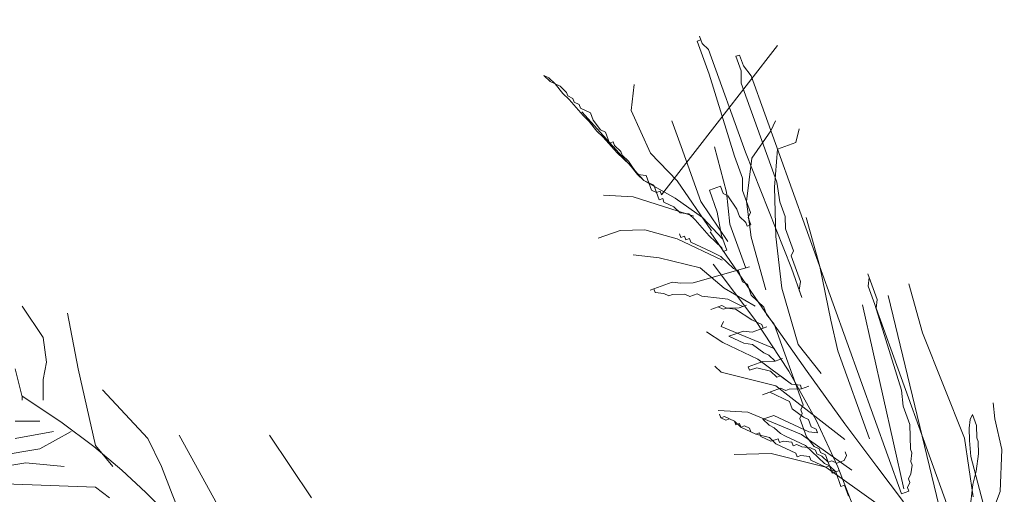
# Model space of a CAD drawing. Units: millimetres. Extents: x 595116 to 630915, y 909473 to 920225.
# Tile 73 of 134: x 629622.585 to 629629.81, y 919282.412 to 919285.898. Entities that reach past the tile are written whole.
import ezdxf

# ---------------------------------------------------------------- set-up
doc = ezdxf.new("R2010")
doc.units = ezdxf.units.MM
doc.layers.add('Dimension', color=3, linetype='Continuous', lineweight=18)
doc.layers.add('L-PLNT', color=85, linetype='Continuous', lineweight=13)
doc.styles.get("Standard").update_dxf_attribs({"font": 'arial.ttf'})
doc.dimstyles.new('ISO-25', dxfattribs={"dimtxt": 9, "dimasz": 6, "dimexe": 1.25, "dimexo": 0.625, "dimtad": 1, "dimlunit": 4, "dimtxsty": 'Standard', "dimcen": 2.5, "dimadec": 0, "dimazin": 0, "dimtfac": 1, "dimtmove": 0, "dimatfit": 3, "dimfxl": 1, "dimarcsym": 0})

# ---------------------------------------------------------------- blocks, each defined once
blk = doc.blocks.new('A$C4FB75ABC')
for p, q in [((2.2354, 4.7176), (2.2283, 4.715)), ((2.238, 4.7104), (2.2329, 4.7248)), ((2.2329, 4.7248), (2.2354, 4.7176)), ((2.1583, 4.4143), (2.3852, 4.7066)), ((2.2283, 4.715), (2.2515, 4.6504)), ((2.2504, 4.6987), (2.238, 4.7104)), ((2.3227, 4.4977), (2.2504, 4.6987)), ((2.3109, 4.688), (2.3037, 4.6854)), ((2.3037, 4.6854), (2.314, 4.6567)), ((2.3186, 4.6665), (2.3109, 4.688)), ((2.3336, 4.6475), (2.3186, 4.6665)), ((1.9382, 4.6431), (1.9285, 4.6477)), ((1.9285, 4.6477), (1.9408, 4.6359)), ((1.9506, 4.6313), (1.9382, 4.6431)), ((2.2515, 4.6504), (2.3011, 4.49)), ((2.314, 4.6567), (2.3146, 4.6326)), ((2.6279, 3.8295), (2.3336, 4.6475)), ((1.9408, 4.6359), (1.9506, 4.6313)), ((1.9603, 4.6267), (1.9506, 4.6313)), ((1.9506, 4.6313), (1.9655, 4.6124)), ((1.9726, 4.6149), (1.9603, 4.6267)), ((2.0989, 4.5793), (2.1049, 4.6301)), ((2.3146, 4.6326), (2.3843, 4.4389)), ((1.9655, 4.6124), (1.9778, 4.6006)), ((1.9752, 4.6078), (1.9726, 4.6149)), ((1.985, 4.6032), (1.9752, 4.6078)), ((1.9876, 4.596), (1.985, 4.6032)), ((1.9778, 4.6006), (2.0051, 4.5699)), ((1.9973, 4.5914), (1.9876, 4.596)), ((1.9999, 4.5842), (1.9973, 4.5914)), ((2.0097, 4.5796), (1.9999, 4.5842)), ((2.1238, 4.4424), (2.0025, 4.577)), ((2.0051, 4.5699), (2.0174, 4.5581)), ((2.0194, 4.575), (2.0097, 4.5796)), ((2.0246, 4.5607), (2.0194, 4.575)), ((2.137, 4.4958), (2.0989, 4.5793)), ((2.0174, 4.5581), (2.0323, 4.5391)), ((2.0395, 4.5417), (2.0246, 4.5607)), ((2.197, 4.5092), (2.1789, 4.5595)), ((2.3723, 4.5399), (2.3815, 4.5594)), ((2.4211, 4.5169), (2.4277, 4.5436)), ((2.0323, 4.5391), (2.0447, 4.5274)), ((2.0493, 4.5371), (2.0395, 4.5417)), ((2.0447, 4.5274), (2.0719, 4.4967)), ((2.057, 4.5156), (2.0493, 4.5371)), ((2.335, 4.486), (2.3723, 4.5399)), ((2.0642, 4.5182), (2.057, 4.5156)), ((2.0668, 4.511), (2.0642, 4.5182)), ((2.0791, 4.4992), (2.0668, 4.511)), ((2.2357, 4.4016), (2.197, 4.5092)), ((2.2859, 4.4197), (2.2621, 4.5084)), ((2.3852, 4.504), (2.4211, 4.5169)), ((2.0719, 4.4967), (2.0966, 4.4731)), ((2.0817, 4.4921), (2.0791, 4.4992)), ((2.094, 4.4803), (2.0817, 4.4921)), ((2.189, 4.4415), (2.137, 4.4958)), ((2.3011, 4.49), (2.3166, 4.4469)), ((2.4125, 4.2707), (2.3227, 4.4977)), ((2.325, 4.4013), (2.335, 4.486)), ((2.3797, 4.4291), (2.3852, 4.504)), ((2.1115, 4.4542), (2.094, 4.4803)), ((2.0966, 4.4731), (2.1115, 4.4542)), ((2.1238, 4.4424), (2.1115, 4.4542)), ((2.1115, 4.4542), (2.1284, 4.4522)), ((2.1284, 4.4522), (2.1336, 4.4378)), ((2.3166, 4.4469), (2.3172, 4.4228)), ((2.1336, 4.4378), (2.1238, 4.4424)), ((2.185, 4.4077), (2.1238, 4.4424)), ((2.1388, 4.4235), (2.1336, 4.4378)), ((2.1336, 4.4378), (2.1434, 4.4332)), ((2.1434, 4.4332), (2.1485, 4.4189)), ((2.2564, 4.3442), (2.189, 4.4415)), ((2.2736, 4.4314), (2.2521, 4.4237)), ((2.2788, 4.4171), (2.2736, 4.4314)), ((2.382, 4.3327), (2.3797, 4.4291)), ((2.3843, 4.4389), (2.3901, 4.4004)), ((2.1029, 4.4105), (2.0449, 4.414)), ((2.222, 4.3723), (2.1029, 4.4105)), ((2.1485, 4.4189), (2.1388, 4.4235)), ((2.1485, 4.4189), (2.1557, 4.4214)), ((2.1537, 4.4045), (2.1485, 4.4189)), ((2.1557, 4.4214), (2.1583, 4.4143)), ((2.2521, 4.4237), (2.2676, 4.3807)), ((2.2885, 4.4125), (2.2788, 4.4171)), ((2.2922, 4.3571), (2.2859, 4.4197)), ((2.306, 4.3864), (2.2885, 4.4125)), ((2.3172, 4.4228), (2.3327, 4.3798)), ((2.1609, 4.4071), (2.1537, 4.4045)), ((2.1634, 4.3999), (2.1609, 4.4071)), ((2.1829, 4.3907), (2.1634, 4.3999)), ((2.1953, 4.379), (2.1829, 4.3907)), ((2.2389, 4.3703), (2.185, 4.4077)), ((2.2882, 4.3232), (2.2357, 4.4016)), ((2.3338, 4.3316), (2.325, 4.4013)), ((2.3901, 4.4004), (2.4004, 4.3717)), ((2.2122, 4.3769), (2.1953, 4.379)), ((2.2245, 4.3652), (2.2122, 4.3769)), ((2.2785, 4.3278), (2.2389, 4.3703)), ((2.2676, 4.3807), (2.2759, 4.335)), ((2.3112, 4.372), (2.306, 4.3864)), ((2.3235, 4.3603), (2.3112, 4.372)), ((2.3327, 4.3798), (2.3281, 4.37)), ((2.3281, 4.37), (2.3333, 4.3557)), ((2.4004, 4.3717), (2.401, 4.3476)), ((2.4678, 4.2744), (2.4414, 4.3703)), ((2.2518, 4.3344), (2.2245, 4.3652)), ((2.3232, 4.271), (2.2922, 4.3571)), ((2.3261, 4.3531), (2.3235, 4.3603)), ((2.3333, 4.3557), (2.3261, 4.3531)), ((2.0779, 4.3448), (2.0349, 4.3293)), ((2.1261, 4.346), (2.0779, 4.3448)), ((2.1893, 4.3282), (2.1261, 4.346)), ((2.1938, 4.3379), (2.1964, 4.3307)), ((2.1964, 4.3307), (2.2036, 4.3333)), ((2.2036, 4.3333), (2.2062, 4.3261)), ((2.2641, 4.3227), (2.2518, 4.3344)), ((2.2538, 4.3417), (2.3557, 4.1924)), ((2.2759, 4.335), (2.2862, 4.3063)), ((2.3628, 4.2285), (2.3338, 4.3316)), ((2.3941, 4.2317), (2.382, 4.3327)), ((2.401, 4.3476), (2.4165, 4.3046)), ((2.277, 4.2868), (2.1893, 4.3282)), ((2.2062, 4.3261), (2.2134, 4.3287)), ((2.2134, 4.3287), (2.2159, 4.3215)), ((2.2159, 4.3215), (2.2354, 4.3124)), ((2.2354, 4.3124), (2.2452, 4.3078)), ((2.2765, 4.3109), (2.2641, 4.3227)), ((2.154, 4.2911), (2.1032, 4.2972)), ((2.2452, 4.3078), (2.255, 4.3032)), ((2.255, 4.3032), (2.2745, 4.294)), ((2.2745, 4.294), (2.2868, 4.2822)), ((2.2791, 4.3037), (2.2765, 4.3109)), ((2.2862, 4.3063), (2.2791, 4.3037)), ((2.4165, 4.3046), (2.4119, 4.2948)), ((2.4119, 4.2948), (2.43, 4.2446)), ((2.234, 4.2713), (2.154, 4.2911)), ((2.3407, 4.1707), (2.2593, 4.2788)), ((2.2868, 4.2822), (2.2991, 4.2704)), ((2.4896, 4.1688), (2.4678, 4.2744)), ((2.2202, 4.242), (2.3304, 4.2736)), ((2.2808, 4.2314), (2.234, 4.2713)), ((2.2991, 4.2704), (2.3089, 4.2658)), ((2.3089, 4.2658), (2.3166, 4.2443)), ((2.4331, 4.2133), (2.4125, 4.2707)), ((2.5803, 4.2095), (2.5622, 4.2597)), ((2.5622, 4.2597), (2.5648, 4.2526)), ((2.1362, 4.228), (2.1792, 4.2435)), ((2.1792, 4.2435), (2.1961, 4.2415)), ((2.1961, 4.2415), (2.2202, 4.242)), ((2.3166, 4.2443), (2.3264, 4.2397)), ((2.3264, 4.2397), (2.3341, 4.2182)), ((2.43, 4.2446), (2.4279, 4.2276)), ((2.5648, 4.2526), (2.5628, 4.2356)), ((2.5628, 4.2356), (2.5757, 4.1997)), ((2.6686, 4.144), (2.6423, 4.2399)), ((2.1434, 4.2306), (2.1362, 4.228)), ((2.1459, 4.2234), (2.1434, 4.2306)), ((2.1629, 4.2214), (2.1459, 4.2234)), ((2.1726, 4.2168), (2.1629, 4.2214)), ((2.1798, 4.2194), (2.1726, 4.2168)), ((2.2039, 4.22), (2.1798, 4.2194)), ((2.2136, 4.2154), (2.2039, 4.22)), ((2.228, 4.2205), (2.2136, 4.2154)), ((2.2377, 4.2159), (2.228, 4.2205)), ((2.2716, 4.2119), (2.2377, 4.2159)), ((2.3419, 4.1967), (2.2808, 4.2314)), ((2.3341, 4.2182), (2.3465, 4.2064)), ((2.4257, 4.1214), (2.3941, 4.2317)), ((2.4279, 4.2276), (2.4331, 4.2133)), ((2.7169, 3.7399), (2.6018, 4.2172)), ((2.2552, 4.1898), (2.2768, 4.1975)), ((2.2885, 4.2099), (2.2716, 4.2119)), ((2.2768, 4.1975), (2.2865, 4.1929)), ((2.308, 4.2007), (2.2885, 4.2099)), ((2.3178, 4.1961), (2.308, 4.2007)), ((2.3106, 4.1935), (2.325, 4.1987)), ((2.325, 4.1987), (2.3178, 4.1961)), ((2.3465, 4.2064), (2.3588, 4.1946)), ((2.6325, 3.8393), (2.5516, 4.1992)), ((2.5757, 4.1997), (2.6279, 4.0321)), ((2.5783, 4.1926), (2.5803, 4.2095)), ((0.9087, 4.1962), (0.9496, 4.1349)), ((0.9973, 4.1826), (1.0177, 4.0736)), ((2.2696, 4.195), (2.2552, 4.1898)), ((2.2793, 4.1904), (2.2696, 4.195)), ((2.2865, 4.1929), (2.2793, 4.1904)), ((2.2865, 4.1929), (2.3106, 4.1935)), ((2.3034, 4.1909), (2.2865, 4.1929)), ((2.3353, 4.17), (2.3034, 4.1909)), ((2.3557, 4.1924), (2.443, 4.0685)), ((2.3588, 4.1946), (2.364, 4.1803)), ((2.364, 4.1803), (2.3789, 4.1614)), ((2.8029, 3.5683), (2.5783, 4.1926)), ((2.2753, 4.1565), (2.2799, 4.1663)), ((2.345, 4.1654), (2.3353, 4.17)), ((2.4072, 4.0691), (2.3407, 4.1707)), ((2.3548, 4.1608), (2.345, 4.1654)), ((2.3574, 4.1536), (2.3548, 4.1608)), ((2.3789, 4.1614), (2.4357, 4.0035)), ((2.5031, 4.1088), (2.4896, 4.1688)), ((2.2785, 4.1252), (2.2466, 4.1462)), ((2.38, 4.1131), (2.2753, 4.1565)), ((2.2902, 4.1376), (2.3189, 4.1479)), ((2.3189, 4.1479), (2.3359, 4.1459)), ((2.3359, 4.1459), (2.3645, 4.1562)), ((2.3645, 4.1562), (2.3574, 4.1536)), ((2.7507, 3.9385), (2.6686, 4.144)), ((0.9496, 4.1349), (0.9564, 4.0872)), ((2.3468, 4.0931), (2.2785, 4.1252)), ((2.3, 4.133), (2.2902, 4.1376)), ((2.3098, 4.1284), (2.3, 4.133)), ((2.3195, 4.1238), (2.3098, 4.1284)), ((2.3364, 4.1218), (2.3195, 4.1238)), ((2.3585, 4.1054), (2.3364, 4.1218)), ((2.4704, 4.0646), (2.4257, 4.1214)), ((2.3683, 4.1008), (2.3585, 4.1054)), ((2.3806, 4.089), (2.3683, 4.1008)), ((2.5651, 3.9366), (2.5031, 4.1088)), ((0.9564, 4.0872), (0.9496, 4.0532)), ((2.3278, 4.0781), (2.3565, 4.0885)), ((2.413, 4.044), (2.3468, 4.0931)), ((2.3565, 4.0885), (2.3806, 4.089)), ((2.3806, 4.089), (2.395, 4.0942)), ((2.395, 4.0942), (2.3806, 4.089)), ((0.8951, 4.0736), (0.9087, 4.0191)), ((1.0177, 4.0736), (1.0518, 3.9238)), ((2.275, 4.0672), (2.2627, 4.079)), ((2.3818, 4.0408), (2.275, 4.0672)), ((2.3304, 4.071), (2.3278, 4.0781)), ((2.3448, 4.0761), (2.3304, 4.071)), ((2.3714, 4.0695), (2.3448, 4.0761)), ((2.3838, 4.0577), (2.3714, 4.0695)), ((2.4608, 3.9732), (2.4072, 4.0691)), ((2.443, 4.0685), (2.5171, 3.9664)), ((0.9496, 4.0532), (0.9496, 4.0123)), ((2.3909, 4.0603), (2.3838, 4.0577)), ((2.413, 4.044), (2.3909, 4.0603)), ((2.43, 4.0419), (2.413, 4.044)), ((1.0654, 4.0327), (1.154, 3.9374)), ((2.3557, 4.0233), (2.3915, 4.0362)), ((2.37, 4.0285), (2.3557, 4.0233)), ((2.3798, 4.0239), (2.37, 4.0285)), ((2.3993, 4.0147), (2.3798, 4.0239)), ((2.5169, 3.9354), (2.3818, 4.0408)), ((2.3915, 4.0362), (2.4013, 4.0316)), ((2.4013, 4.0316), (2.4084, 4.0342)), ((2.4084, 4.0342), (2.4325, 4.0348)), ((2.4325, 4.0348), (2.43, 4.0419)), ((2.4325, 4.0348), (2.4469, 4.0399)), ((2.4469, 4.0399), (2.4325, 4.0348)), ((2.6279, 4.0321), (2.6311, 4.0008)), ((0.9842, 3.9699), (0.9085, 4.0207)), ((0.9087, 4.0191), (0.9087, 4.0123)), ((2.409, 4.0101), (2.3993, 4.0147)), ((2.4142, 3.9957), (2.409, 4.0101)), ((2.8101, 3.9761), (2.8069, 4.0074)), ((2.3275, 3.9889), (2.2696, 3.9923)), ((2.2748, 3.978), (2.2722, 3.9852)), ((2.2722, 3.9852), (2.2748, 3.978)), ((2.4323, 3.9455), (2.3275, 3.9889)), ((2.4363, 3.9794), (2.4142, 3.9957)), ((2.4337, 3.9866), (2.4291, 3.9768)), ((2.4357, 4.0035), (2.4311, 3.9937)), ((2.4311, 3.9937), (2.4337, 3.9866)), ((2.6311, 4.0008), (2.644, 3.965)), ((0.8951, 3.9715), (0.9428, 3.9715)), ((1.0487, 3.9217), (0.9842, 3.9699)), ((2.2748, 3.978), (2.2819, 3.9806)), ((2.2845, 3.9734), (2.2748, 3.978)), ((2.2819, 3.9806), (2.2917, 3.976)), ((2.2917, 3.976), (2.2845, 3.9734)), ((2.3014, 3.9714), (2.2917, 3.976)), ((2.2917, 3.976), (2.3014, 3.9714)), ((2.304, 3.9642), (2.3014, 3.9714)), ((2.3014, 3.9714), (2.3138, 3.9596)), ((2.3112, 3.9668), (2.304, 3.9642)), ((2.3138, 3.9596), (2.3112, 3.9668)), ((2.3568, 3.9751), (2.3783, 3.9828)), ((2.3691, 3.9633), (2.3568, 3.9751)), ((2.3783, 3.9828), (2.3881, 3.9782)), ((2.3881, 3.9782), (2.4076, 3.9691)), ((2.4076, 3.9691), (2.4173, 3.9645)), ((2.4291, 3.9768), (2.442, 3.9409)), ((2.446, 3.9748), (2.4363, 3.9794)), ((2.4512, 3.9604), (2.446, 3.9748)), ((2.5035, 3.8821), (2.4608, 3.9732)), ((2.5171, 3.9664), (2.5794, 3.8826)), ((2.7619, 3.975), (2.7599, 3.958)), ((2.7665, 3.9847), (2.7619, 3.975)), ((2.7742, 3.9632), (2.7665, 3.9847)), ((2.8236, 3.9161), (2.8101, 3.9761)), ((0.97, 3.951), (0.8951, 3.9374)), ((1.0041, 3.951), (0.9428, 3.917)), ((2.3209, 3.9622), (2.3138, 3.9596)), ((2.3138, 3.9596), (2.3235, 3.955)), ((2.3307, 3.9576), (2.3209, 3.9622)), ((2.3235, 3.955), (2.3333, 3.9504)), ((2.3333, 3.9504), (2.3307, 3.9576)), ((2.343, 3.9458), (2.3333, 3.9504)), ((2.3333, 3.9504), (2.343, 3.9458)), ((2.3502, 3.9484), (2.343, 3.9458)), ((2.3528, 3.9412), (2.3502, 3.9484)), ((2.3789, 3.9587), (2.3691, 3.9633)), ((2.3912, 3.947), (2.3789, 3.9587)), ((2.401, 3.9424), (2.3912, 3.947)), ((2.4173, 3.9645), (2.4368, 3.9553)), ((2.4368, 3.9553), (2.4466, 3.9507)), ((2.4466, 3.9507), (2.4635, 3.9487)), ((2.4609, 3.9558), (2.4512, 3.9604)), ((2.4635, 3.9487), (2.4609, 3.9558)), ((2.644, 3.965), (2.6451, 3.9167)), ((2.7599, 3.958), (2.7605, 3.9339)), ((2.7748, 3.9391), (2.7742, 3.9632)), ((1.154, 3.9374), (1.1812, 3.8829)), ((1.2153, 3.9442), (1.2902, 3.808)), ((1.3924, 3.9442), (1.4742, 3.8217)), ((2.343, 3.9458), (2.3697, 3.9392)), ((2.3723, 3.932), (2.3528, 3.9412)), ((2.3697, 3.9392), (2.3821, 3.9274)), ((2.3866, 3.9372), (2.3723, 3.932)), ((2.3821, 3.9274), (2.3918, 3.9228)), ((2.3892, 3.93), (2.3866, 3.9372)), ((2.3964, 3.9326), (2.3892, 3.93)), ((2.4133, 3.9306), (2.3964, 3.9326)), ((2.44, 3.924), (2.401, 3.9424)), ((2.4159, 3.9234), (2.4133, 3.9306)), ((2.5304, 3.8755), (2.4323, 3.9455)), ((2.442, 3.9409), (2.4569, 3.922)), ((2.7679, 3.8231), (2.7507, 3.9385)), ((2.7605, 3.9339), (2.7636, 3.9026)), ((2.7774, 3.9319), (2.7748, 3.9391)), ((2.778, 3.9078), (2.7774, 3.9319)), ((0.9428, 3.917), (0.861, 3.9034)), ((1.1035, 3.8758), (1.0487, 3.9217)), ((1.0518, 3.9238), (1.0858, 3.8829)), ((2.3729, 3.9079), (2.3006, 3.9062)), ((2.4796, 3.8815), (2.3729, 3.9079)), ((2.3918, 3.9228), (2.4113, 3.9137)), ((2.4113, 3.9137), (2.4211, 3.9091)), ((2.4231, 3.926), (2.4159, 3.9234)), ((2.4211, 3.9091), (2.4237, 3.9019)), ((2.4328, 3.9214), (2.4231, 3.926)), ((2.4498, 3.9194), (2.4328, 3.9214)), ((2.4523, 3.9122), (2.44, 3.924)), ((2.4595, 3.9148), (2.4498, 3.9194)), ((2.477, 3.8887), (2.4523, 3.9122)), ((2.4569, 3.922), (2.4667, 3.9174)), ((2.4621, 3.9076), (2.4595, 3.9148)), ((2.4667, 3.9174), (2.4693, 3.9102)), ((2.4693, 3.9102), (2.479, 3.9056)), ((2.5175, 3.9113), (2.52, 3.9042)), ((2.6451, 3.9167), (2.6477, 3.9096)), ((2.6477, 3.9096), (2.6457, 3.8926)), ((2.8207, 3.834), (2.8236, 3.9161)), ((0.9155, 3.8897), (0.8338, 3.8761)), ((0.9905, 3.8829), (0.9155, 3.8897)), ((2.4237, 3.9019), (2.4308, 3.9045)), ((2.4308, 3.9045), (2.4478, 3.9025)), ((2.4478, 3.9025), (2.4503, 3.8953)), ((2.4503, 3.8953), (2.4698, 3.8861)), ((2.4718, 3.903), (2.4621, 3.9076)), ((2.4842, 3.8913), (2.4718, 3.903)), ((2.4868, 3.8841), (2.477, 3.8887)), ((2.479, 3.9056), (2.4868, 3.8841)), ((2.4914, 3.8938), (2.4842, 3.8913)), ((2.5011, 3.8892), (2.4914, 3.8938)), ((2.5155, 3.8944), (2.5011, 3.8892)), ((2.52, 3.9042), (2.5155, 3.8944)), ((2.6457, 3.8926), (2.6483, 3.8855)), ((2.7636, 3.9026), (2.8247, 3.6653)), ((2.7739, 3.8739), (2.778, 3.9078)), ((1.1506, 3.8319), (1.1035, 3.8758)), ((1.1812, 3.8829), (1.2017, 3.8285)), ((2.4698, 3.8861), (2.4796, 3.8815)), ((2.4796, 3.8815), (2.4868, 3.8841)), ((2.5777, 3.8114), (2.4796, 3.8815)), ((2.4868, 3.8841), (2.4893, 3.8769)), ((2.4919, 3.8697), (2.4868, 3.8841)), ((2.4868, 3.8841), (2.4991, 3.8723)), ((2.4893, 3.8769), (2.4991, 3.8723)), ((2.5063, 3.8749), (2.4919, 3.8697)), ((2.4991, 3.8723), (2.5063, 3.8749)), ((2.4991, 3.8723), (2.5094, 3.8436)), ((2.5372, 3.7949), (2.5035, 3.8821)), ((2.5794, 3.8826), (2.6314, 3.8136)), ((2.6483, 3.8855), (2.6463, 3.8685)), ((2.7673, 3.8473), (2.7739, 3.8739)), ((2.6443, 3.8516), (2.6397, 3.8418)), ((2.6463, 3.8685), (2.6417, 3.8588)), ((2.6417, 3.8588), (2.6443, 3.8516)), ((0.8746, 3.8489), (1.0518, 3.8421)), ((1.0518, 3.8421), (1.079, 3.8217)), ((1.1917, 3.7897), (1.1506, 3.8319)), ((2.5094, 3.8436), (2.5166, 3.8462)), ((2.5166, 3.8462), (2.5244, 3.8247)), ((2.6423, 3.8347), (2.6279, 3.8295)), ((2.6397, 3.8418), (2.6423, 3.8347)), ((2.7653, 3.8303), (2.7673, 3.8473)), ((2.7957, 3.7683), (2.8207, 3.834)), ((1.2017, 3.8285), (1.2153, 3.7944)), ((2.7613, 3.7965), (2.7653, 3.8303))]:
    blk.add_line(p, q)
blk = doc.blocks.new('*D216')
at = {"layer": 'Defpoints', "color": 0, "transparency": 16777216}
for p in [(629743.5408, 919411.9276), (629505.0408, 919411.8279), (629743.5408, 918832.3776)]:
    blk.add_point(p, dxfattribs=at)
at = {"layer": 'Dimension', "color": 0, "lineweight": -2, "transparency": 16777216}
for p, q in [((629743.5408, 919411.3026), (629743.5408, 918831.1276)), ((629505.0408, 919411.2029), (629505.0408, 918831.1276)), ((629511.0408, 918832.3776), (629737.5408, 918832.3776))]:
    blk.add_line(p, q, dxfattribs=at)
at = {"layer": 'Dimension', "color": 0, "transparency": 16777216}
for points in [[(629511.0408, 918833.3776), (629511.0408, 918831.3776), (629505.0408, 918832.3776)], [(629737.5408, 918833.3776), (629737.5408, 918831.3776), (629743.5408, 918832.3776)]]:
    blk.add_solid(points, dxfattribs=at)
at = {"layer": 'Dimension', "color": 0, "transparency": 16777216, "insert": (629624.2908, 918837.656), "char_height": 9, "attachment_point": 5}
blk.add_mtext('19\'-10 1/2"', dxfattribs=at)

msp = doc.modelspace()

# ---------------------------------------------------------------- block references
at = {"layer": 'L-PLNT', "xscale": 3.753413438031968, "yscale": 3.753413438031968, "zscale": 3.753413438031968}
msp.add_blockref('A$C4FB75ABC', (629619.1929, 919268.043), dxfattribs=at)

# ---------------------------------------------------------------- dimensions: what is measured, and where the dimension line sits
at = {"layer": 'Dimension'}
dim = msp.add_linear_dim(base=(629743.5408, 918832.3776), p1=(629505.0408, 919411.8279), p2=(629743.5408, 919411.9276), dimstyle='ISO-25', override={"dimdec": 1, "dimlfac": 1, "dimrnd": 0, "dimzin": 1, "dimdsep": 46, "dimlunit": 4, "dimfrac": 2}, dxfattribs=at)
dim.commit()
dim.dimension.update_dxf_attribs({"geometry": '*D216', "text_midpoint": (629624.2908, 918837.656)})

doc.saveas('drawing.dxf')
